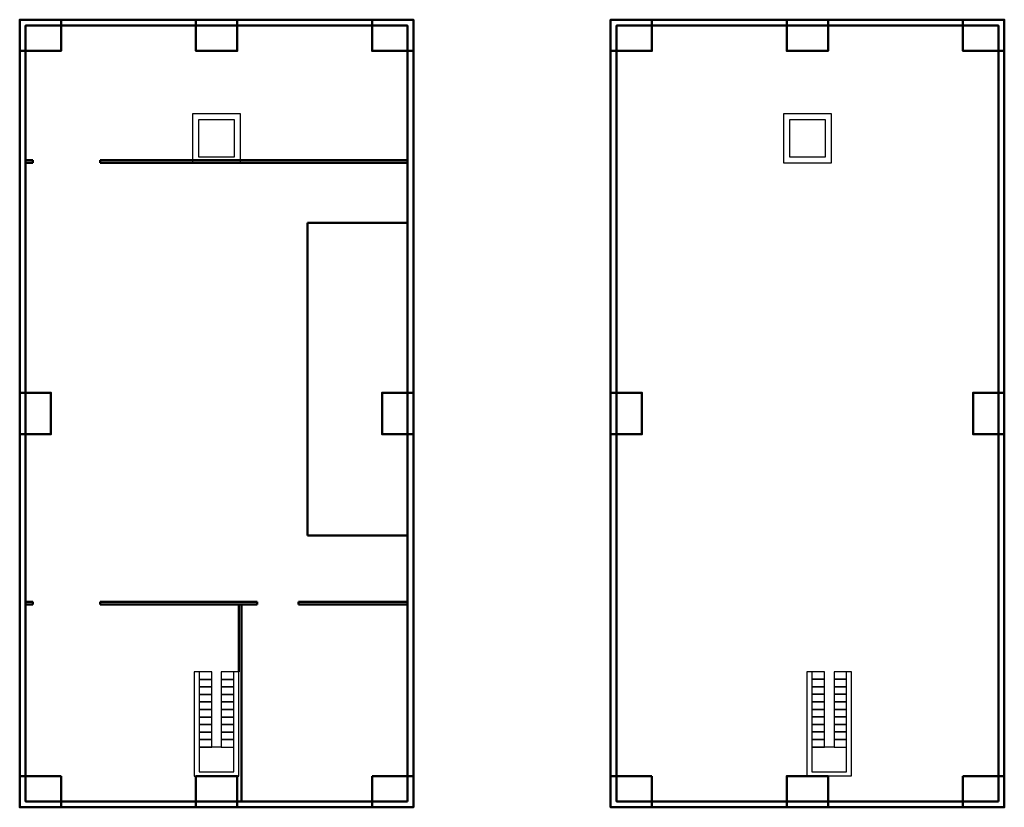
# Model space of a CAD drawing. Units: feet. Extents: x 1080 to 13444, y 870 to 7060.
# Tile 4 of 5: x 7629 to 9130, y 1047 to 2247. Entities that reach past the tile are written whole.
import ezdxf

# ---------------------------------------------------------------- set-up
doc = ezdxf.new("R2010")
doc.units = ezdxf.units.FT
for name, color, linetype, lineweight in [('A-COLS', 1, 'Continuous', 50), ('A-FLOR-EVTR', 6, 'Continuous', 25), ('A-FLOR-STRS', 2, 'Continuous', 25), ('A-WALL', 7, 'Continuous', 50)]:
    doc.layers.add(name, color=color, linetype=linetype, lineweight=lineweight)

msp = doc.modelspace()

# ---------------------------------------------------------------- linework, layer by layer
at = {"layer": 'A-COLS'}
for points in [[(7628.8, 2246.8), (7691.8, 2246.8), (7691.8, 2199.1), (7628.8, 2199.1)], [(7897.3, 2246.8), (7960.3, 2246.8), (7960.3, 2199.1), (7897.3, 2199.1)], [(8165.8, 2246.8), (8228.8, 2246.8), (8228.8, 2199.1), (8165.8, 2199.1)], [(8529.5, 2246.8), (8592.5, 2246.8), (8592.5, 2199.1), (8529.5, 2199.1)], [(8798, 2246.8), (8861, 2246.8), (8861, 2199.1), (8798, 2199.1)], [(9066.5, 2246.8), (9129.5, 2246.8), (9129.5, 2199.1), (9066.5, 2199.1)], [(7628.8, 1615.2), (7628.8, 1678.3), (7676.4, 1678.3), (7676.4, 1615.2)], [(8228.8, 1678.3), (8228.8, 1615.2), (8181.1, 1615.2), (8181.1, 1678.3)], [(8529.5, 1615.2), (8529.5, 1678.3), (8577.1, 1678.3), (8577.1, 1615.2)], [(9129.5, 1678.3), (9129.5, 1615.2), (9081.9, 1615.2), (9081.9, 1678.3)], [(7691.8, 1094.4), (7628.8, 1094.4), (7628.8, 1046.8), (7691.8, 1046.8)], [(7960.3, 1046.8), (7897.3, 1046.8), (7897.3, 1094.4), (7960.3, 1094.4)], [(8165.8, 1094.4), (8228.8, 1094.4), (8228.8, 1046.8), (8165.8, 1046.8)], [(8592.5, 1094.4), (8529.5, 1094.4), (8529.5, 1046.8), (8592.5, 1046.8)], [(8861, 1046.8), (8798, 1046.8), (8798, 1094.4), (8861, 1094.4)], [(9066.5, 1094.4), (9129.5, 1094.4), (9129.5, 1046.8), (9066.5, 1046.8)]]:
    msp.add_lwpolyline(points, close=True, dxfattribs=at)
at = {"layer": 'A-FLOR-EVTR'}
for points in [[(7892.1, 2028.8), (7965.4, 2028.8), (7965.4, 2103.4), (7892.1, 2103.4), (7892.1, 2101.1)], [(8792.9, 2028.8), (8866.2, 2028.8), (8866.2, 2103.4), (8792.9, 2103.4), (8792.9, 2101.1)], [(7901.2, 2037.8), (7956.3, 2037.8), (7956.3, 2094.3), (7901.2, 2094.3)], [(8802, 2037.8), (8857.1, 2037.8), (8857.1, 2094.3), (8802, 2094.3)]]:
    msp.add_lwpolyline(points, close=True, dxfattribs=at)
at = {"layer": 'A-FLOR-STRS'}
for points in [[(7902.3, 1253.1), (7894.7, 1253.1), (7894.7, 1094.4), (7962.8, 1094.4), (7962.8, 1253.1), (7955.2, 1253.1)], [(8836.3, 1253.3), (8828.7, 1253.3), (8828.7, 1094.5), (8896.8, 1094.5), (8896.8, 1253.3), (8889.2, 1253.3)], [(7936.1, 1138.5), (7902.3, 1138.5), (7902.3, 1100.6), (7955.2, 1100.6), (7955.2, 1138.5)], [(8870.1, 1138.6), (8836.3, 1138.6), (8836.3, 1100.7), (8889.2, 1100.7), (8889.2, 1138.6)]]:
    msp.add_lwpolyline(points, dxfattribs=at)
for points in [[(7902.3, 1253.1), (7902.3, 1241.7), (7921.4, 1241.7), (7921.4, 1253.1)], [(7936.1, 1253.1), (7936.1, 1241.7), (7955.2, 1241.7), (7955.2, 1253.1)], [(8836.3, 1253.3), (8836.3, 1241.8), (8855.4, 1241.8), (8855.4, 1253.3)], [(8870.1, 1253.3), (8870.1, 1241.8), (8889.2, 1241.8), (8889.2, 1253.3)], [(7902.3, 1241.7), (7902.3, 1230.2), (7921.4, 1230.2), (7921.4, 1241.7)], [(7936.1, 1241.7), (7936.1, 1230.2), (7955.2, 1230.2), (7955.2, 1241.7)], [(8836.3, 1241.8), (8836.3, 1230.3), (8855.4, 1230.3), (8855.4, 1241.8)], [(8870.1, 1241.8), (8870.1, 1230.3), (8889.2, 1230.3), (8889.2, 1241.8)], [(7902.3, 1230.2), (7902.3, 1218.7), (7921.4, 1218.7), (7921.4, 1230.2)], [(7902.3, 1218.7), (7902.3, 1207.3), (7921.4, 1207.3), (7921.4, 1218.7)], [(7936.1, 1230.2), (7936.1, 1218.7), (7955.2, 1218.7), (7955.2, 1230.2)], [(7936.1, 1218.7), (7936.1, 1207.3), (7955.2, 1207.3), (7955.2, 1218.7)], [(8836.3, 1230.3), (8836.3, 1218.9), (8855.4, 1218.9), (8855.4, 1230.3)], [(8836.3, 1218.9), (8836.3, 1207.4), (8855.4, 1207.4), (8855.4, 1218.9)], [(8870.1, 1230.3), (8870.1, 1218.9), (8889.2, 1218.9), (8889.2, 1230.3)], [(8870.1, 1218.9), (8870.1, 1207.4), (8889.2, 1207.4), (8889.2, 1218.9)], [(7902.3, 1207.3), (7902.3, 1195.8), (7921.4, 1195.8), (7921.4, 1207.3)], [(7936.1, 1207.3), (7936.1, 1195.8), (7955.2, 1195.8), (7955.2, 1207.3)], [(8836.3, 1207.4), (8836.3, 1195.9), (8855.4, 1195.9), (8855.4, 1207.4)], [(8870.1, 1207.4), (8870.1, 1195.9), (8889.2, 1195.9), (8889.2, 1207.4)], [(7902.3, 1195.8), (7902.3, 1184.3), (7921.4, 1184.3), (7921.4, 1195.8)], [(7936.1, 1195.8), (7936.1, 1184.3), (7955.2, 1184.3), (7955.2, 1195.8)], [(8836.3, 1195.9), (8836.3, 1184.5), (8855.4, 1184.5), (8855.4, 1195.9)], [(8870.1, 1195.9), (8870.1, 1184.5), (8889.2, 1184.5), (8889.2, 1195.9)], [(7902.3, 1184.3), (7902.3, 1172.9), (7921.4, 1172.9), (7921.4, 1184.3)], [(7902.3, 1172.9), (7902.3, 1161.4), (7921.4, 1161.4), (7921.4, 1172.9)], [(7936.1, 1184.3), (7936.1, 1172.9), (7955.2, 1172.9), (7955.2, 1184.3)], [(7936.1, 1172.9), (7936.1, 1161.4), (7955.2, 1161.4), (7955.2, 1172.9)], [(8836.3, 1184.5), (8836.3, 1173), (8855.4, 1173), (8855.4, 1184.5)], [(8836.3, 1173), (8836.3, 1161.5), (8855.4, 1161.5), (8855.4, 1173)], [(8870.1, 1184.5), (8870.1, 1173), (8889.2, 1173), (8889.2, 1184.5)], [(8870.1, 1173), (8870.1, 1161.5), (8889.2, 1161.5), (8889.2, 1173)], [(7902.3, 1161.4), (7902.3, 1149.9), (7921.4, 1149.9), (7921.4, 1161.4)], [(7936.1, 1161.4), (7936.1, 1149.9), (7955.2, 1149.9), (7955.2, 1161.4)], [(8836.3, 1161.5), (8836.3, 1150.1), (8855.4, 1150.1), (8855.4, 1161.5)], [(8870.1, 1161.5), (8870.1, 1150.1), (8889.2, 1150.1), (8889.2, 1161.5)], [(7902.3, 1149.9), (7902.3, 1138.5), (7921.4, 1138.5), (7921.4, 1149.9)], [(7936.1, 1149.9), (7936.1, 1138.5), (7955.2, 1138.5), (7955.2, 1149.9)], [(8836.3, 1150.1), (8836.3, 1138.6), (8855.4, 1138.6), (8855.4, 1150.1)], [(8870.1, 1150.1), (8870.1, 1138.6), (8889.2, 1138.6), (8889.2, 1150.1)]]:
    msp.add_lwpolyline(points, close=True, dxfattribs=at)
at = {"layer": 'A-WALL'}
for p, q in [((7637.8, 2032.8), (7649, 2032.8)), ((7637.8, 2028.8), (7649, 2028.8)), ((7649, 2028.8), (7649, 2032.8)), ((7751.6, 2032.8), (7751.6, 2028.8)), ((7751.6, 2032.8), (8219.8, 2032.8)), ((7751.6, 2028.8), (8219.8, 2028.8)), ((8219.8, 1937.5), (8067.4, 1937.5)), ((8067.4, 1937.5), (8067.4, 1460.8)), ((8067.4, 1460.8), (8219.8, 1460.8)), ((7637.8, 1359.6), (7649, 1359.6)), ((7637.8, 1355.6), (7649, 1355.6)), ((7649, 1355.6), (7649, 1359.6)), ((7751.6, 1359.6), (7751.6, 1355.6)), ((7751.6, 1359.6), (7990.8, 1359.6)), ((7751.6, 1355.6), (7990.8, 1355.6)), ((7962.8, 1253.1), (7962.8, 1355.6)), ((7966.8, 1055.8), (7966.8, 1355.6)), ((7990.8, 1355.6), (7990.8, 1359.6)), ((8053.9, 1359.6), (8053.9, 1355.6)), ((8053.9, 1359.6), (8219.8, 1359.6)), ((8053.9, 1355.6), (8219.8, 1355.6))]:
    msp.add_line(p, q, dxfattribs=at)
for points in [[(8228.8, 1046.8), (7628.8, 1046.8), (7628.8, 2246.8), (8228.8, 2246.8)], [(8219.8, 1055.8), (7637.8, 1055.8), (7637.8, 2237.8), (8219.8, 2237.8)], [(9129.5, 1046.8), (8529.5, 1046.8), (8529.5, 2246.8), (9129.5, 2246.8)], [(9120.5, 1055.8), (8538.5, 1055.8), (8538.5, 2237.8), (9120.5, 2237.8)]]:
    msp.add_lwpolyline(points, close=True, dxfattribs=at)

doc.saveas('drawing.dxf')
